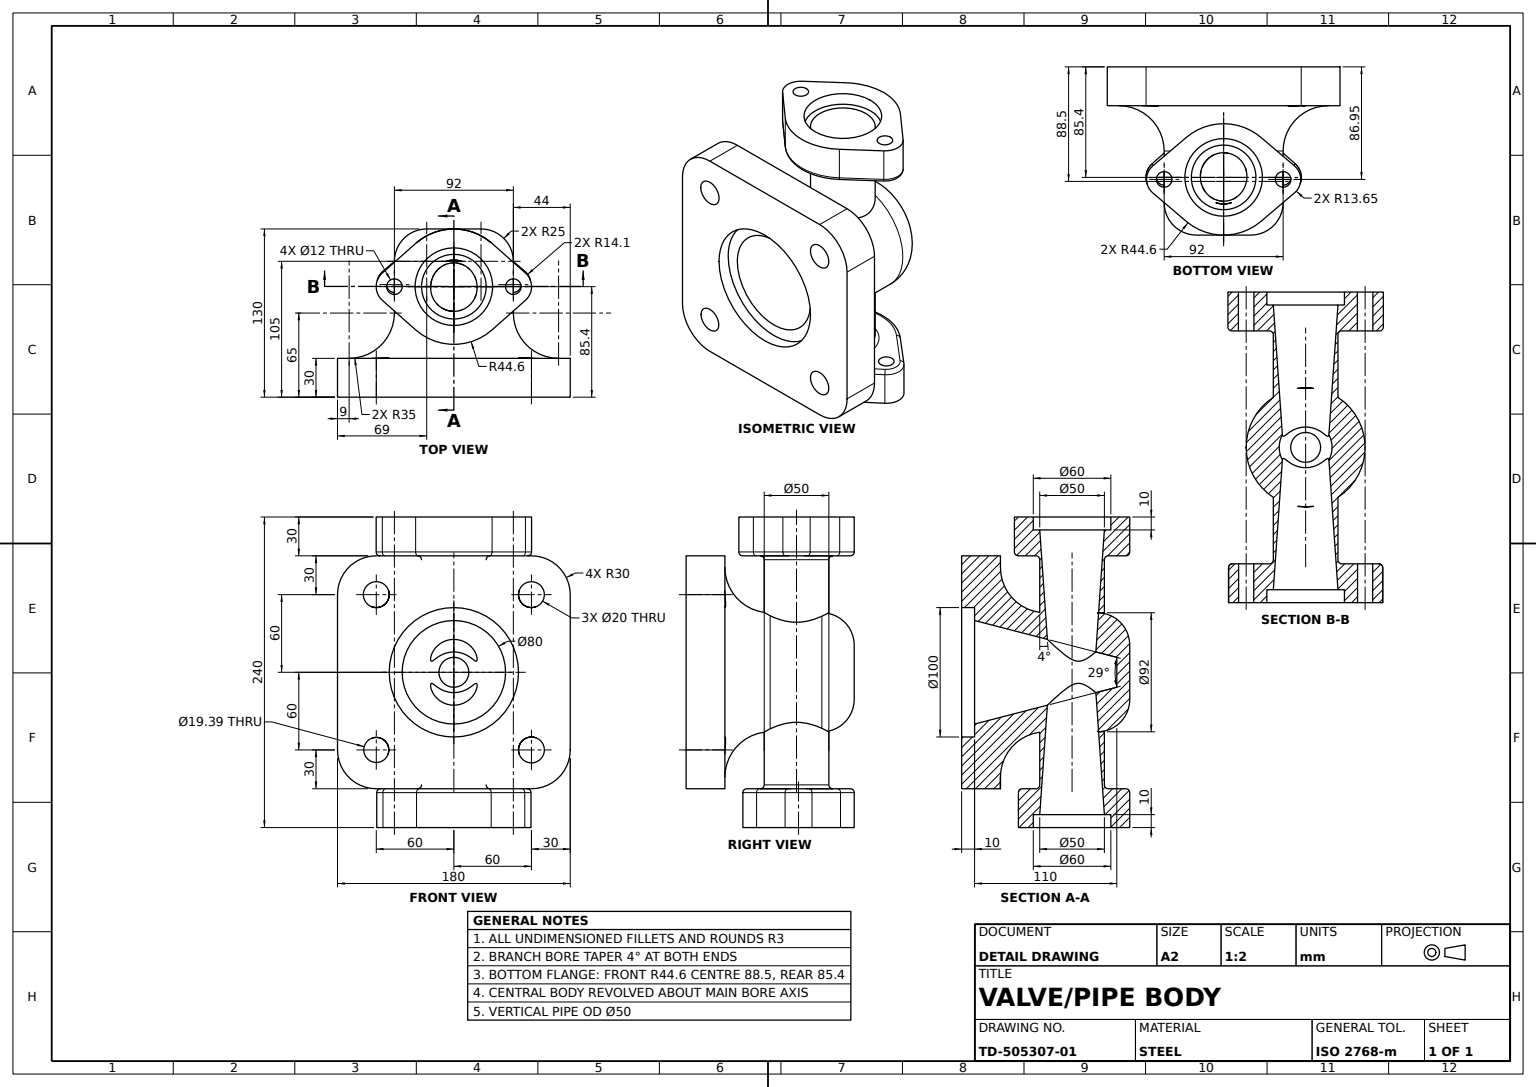
SolidWorks part; units mm, degrees
material "Plain Carbon Steel"
ref_plane "Front Plane" through (0, 0, 0) normal (0, 0, 1) x (1, 0, 0)
ref_plane "Top Plane" through (0, 0, 0) normal (0, 1, 0) x (1, 0, 0)
ref_plane "Right Plane" through (0, 0, 0) normal (1, 0, 0) x (0, 0, -1)
sketch "Square Flange Sketch" plane through (0, 0, 0) normal (0, 0, 1) x (1, 0, 0)
  line L1 (-90, 90) -> (90, 90)
  line L2 (-90, 90) -> (-90, -90)
  line L3 (-90, -90) -> (90, -90)
  line L4 (90, 90) -> (90, -90)
  line L5 (-90, 90) -> (90, -90) construction
  line L6 (-90, -90) -> (90, 90) construction
  point P0 (0, 0)
  dimension "D1" = 180
  dimension "D2" = 180
extrude "Square Flange 180x180" add sketch "Square Flange Sketch" along normal blind 30
fillet "Flange Corner Fillets R30" radius 30 4 edges at (-90, -90, 15) (90, -90, 15) (-90, 90, 15) (90, 90, 15)
sketch "Tee Body Profile Sketch" plane through (0, 0, 0) normal (0, 1, 0) x (1, 0, 0)
  line L0 (0, 100) -> (0, 0) construction
  line L1 (0, 100) -> (21, 100)
  line L2 (46, 75) -> (46, 35)
  line L3 (0, 0) -> (81, 0)
  line L4 (0, 100) -> (0, 0)
  arc A0 (46, 75) -> (21, 100) centre (21, 75) ccw
  arc A1 (46, 35) -> (81, 0) centre (81, 35) ccw
  dimension "D2" = 25
  dimension "D4" = 35
  dimension "D1" = 100
  dimension "D3" = 46
revolve "Tee Body Revolve" add sketch "Tee Body Profile Sketch" angle 360 about L0
sketch "Oval Flange A Sketch" plane through (0, -90, 0) normal (0, -1, 0) x (1, 0, 0)
  line L0 (0, -113.6555) -> (0, 0) construction
  line L1 (73.4602, -56.9504) -> (-69.6808, -56.9504) construction
  line L2 (-28.8618, -24.4984) -> (-54.8334, -46.5436)
  line L3 (-54.8334, -67.3571) -> (-28.8618, -89.4023)
  line L4 (28.8618, -89.4023) -> (54.8334, -67.3571)
  line L5 (54.8334, -46.5436) -> (28.8618, -24.4984)
  arc A0 (28.8618, -89.4023) -> (-28.8618, -89.4023) centre (0, -55.4) cw
  arc A1 (-28.8618, -24.4984) -> (28.8618, -24.4984) centre (0, -58.5007) cw
  arc A2 (54.8334, -67.3571) -> (54.8334, -46.5436) centre (46, -56.9504) ccw
  arc A3 (-54.8334, -67.3571) -> (-54.8334, -46.5436) centre (-46, -56.9504) cw
  circle A4 centre (-46, -56.9504) radius 6
  circle A5 centre (46, -56.9504) radius 6
  point P10 (0, -113.9007)
  point P16 (67.0937, -56.9504)
  point P19 (-67.0937, -56.9504)
  point P20 (0, -100)
  dimension "D1" = 44.6
  dimension "D2" = 13.6502
  dimension "D5" = 12
  dimension "D6" = 12
  dimension "D3" = 92
  dimension "D4" = 100
extrude "Oval Flange A" add sketch "Oval Flange A Sketch" along normal blind 30 separate body
sketch "Oval Flange B Sketch" plane through (0, 90, 0) normal (0, 1, 0) x (1, 0, 0)
  line L0 (0, 109.9701) -> (0, 0) construction
  line L1 (110.9056, 55.4) -> (-68.1303, 55.4) construction
  line L2 (29.5717, 88.7867) -> (55.3489, 65.955)
  line L3 (55.3489, 44.845) -> (29.5717, 22.0133)
  line L4 (-29.5717, 22.0133) -> (-55.3489, 44.845)
  line L5 (-55.3489, 65.955) -> (-29.5717, 88.7867)
  arc A0 (29.5717, 22.0133) -> (-29.5717, 22.0133) centre (0, 55.4) cw
  arc A1 (-29.5717, 88.7867) -> (29.5717, 88.7867) centre (0, 55.4) cw
  arc A2 (55.3489, 44.845) -> (55.3489, 65.955) centre (46, 55.4) ccw
  arc A3 (-55.3489, 65.955) -> (-55.3489, 44.845) centre (-46, 55.4) ccw
  circle A4 centre (-46, 55.4) radius 6
  circle A5 centre (46, 55.4) radius 6
  point P11 (0, -4.1794)
  point P14 (0, 114.9794)
  point P17 (67.2656, 55.4)
  point P20 (-67.2656, 55.4)
  point P25 (0, 100)
  dimension "D1" = 44.6
  dimension "D2" = 14.1
  dimension "D5" = 12
  dimension "D6" = 12
  dimension "D3" = 100
  dimension "D4" = 92
extrude "Oval Flange B" add sketch "Oval Flange B Sketch" along normal blind 30 separate body
sketch "Flange B Counterbore Sketch" plane through (0, 120, 0) normal (0, 1, 0) x (1, 0, 0)
  circle A0 centre (0, 55.4) radius 30
  dimension "D1" = 60
extrude "Flange B Counterbore Ø60" cut sketch "Flange B Counterbore Sketch" against normal blind 10
sketch "Flange A Counterbore Sketch" plane through (0, -120, 0) normal (0, -1, 0) x (1, 0, 0)
  circle A0 centre (0, -55.4) radius 30
  dimension "D1" = 60
extrude "Flange A Counterbore Ø60" cut sketch "Flange A Counterbore Sketch" against normal blind 10
sketch "Main Port Counterbore Sketch" plane through (0, 0, 30) normal (0, 0, 1) x (1, 0, 0)
  circle A0 centre (0, 0) radius 50
  dimension "D1" = 100
extrude "Main Port Counterbore Ø100" cut sketch "Main Port Counterbore Sketch" against normal blind 10
sketch "Main Bore Sketch" plane through (0, 0, 20) normal (0, 0, 1) x (1, 0, 0)
  circle A0 centre (0, 0) radius 40
  dimension "D1" = 80
extrude "Main Tapered Bore Ø80" cut sketch "Main Bore Sketch" against normal blind 110 draft 14.5
sketch "Branch Neck B Sketch" plane through (0, 90, 0) normal (0, -1, 0) x (1, 0, 0)
  circle A0 centre (0, -55.4) radius 25
  dimension "D1" = 50
extrude "Branch Neck B Ø50" add sketch "Branch Neck B Sketch" along normal up to surface (44 mm away)
sketch "Branch Neck A Sketch" plane through (0, -90, 0) normal (0, 1, 0) x (1, 0, 0)
  circle A0 centre (0, 55.4) radius 25
  dimension "D1" = 50
extrude "Branch Neck A Ø50" add sketch "Branch Neck A Sketch" along normal up to surface (44 mm away)
sketch "Branch Bore B Sketch" plane through (0, 110, 0) normal (0, 1, 0) x (1, 0, 0)
  circle A0 centre (0, 55.4) radius 25
  dimension "D1" = 50
extrude "Branch Tapered Bore B Ø50" cut sketch "Branch Bore B Sketch" against normal blind 110 draft 4
sketch "Branch Bore A Sketch" plane through (0, -110, 0) normal (0, -1, 0) x (1, 0, 0)
  circle A0 centre (0, -55.4) radius 25
  dimension "D1" = 50
extrude "Branch Tapered Bore A Ø50" cut sketch "Branch Bore A Sketch" against normal blind 110 draft 4
fillet "Oval Flange Fillets R3" radius 3 16 edges at (-41.8476, -90, -78.3797) (-59.6502, -90, -56.9504) (-41.8476, -90, -35.521) (0, -90, -13.9007) (41.8476, -90, -35.521) (59.6502, -90, -56.9504) (41.8476, -90, -78.3797) (42.4603, 90, -77.3708) (60.1, 90, -55.4) (42.4603, 90, -33.4292) (0, 90, -10.8) (-42.4603, 90, -33.4292) (-60.1, 90, -55.4) (-42.4603, 90, -77.3708) (0, -90, -100) (0, 90, -100)
fillet "Branch Neck Fillets R3" radius 3 2 edges at (0, -90, -30.4) (0, 90, -80.4)
sketch "Relief Cut 12x12 Sketch" plane through (0, 0, 30) normal (0, 0, 1) x (1, 0, 0)
  line L0 (0, 90) -> (0, -90) construction
  line L1 (-27.5826, 90) -> (27.5826, 90) construction
  line L2 (-60, -90) -> (60, -90) construction
  line L3 (90, 0) -> (-90, 0) construction
  line L4 (90, -60) -> (90, 60) construction
  line L5 (-90, 60) -> (-90, -60) construction
  circle A0 centre (-60, 60) radius 6
  circle A1 centre (60, 60) radius 6
  circle A2 centre (60, -60) radius 6
  circle A3 centre (-60, -60) radius 6
  dimension "D1" = 12
  dimension "D2" = 12
extrude "Relief Cut 12x12" cut sketch "Relief Cut 12x12 Sketch" against normal blind 15
sketch "Relief Cut 20x20 Sketch" plane through (0, 0, 30) normal (0, 0, 1) x (1, 0, 0)
  circle A0 centre (-60, 60) radius 10
  circle A1 centre (60, 60) radius 10
  circle A2 centre (-60, -60) radius 9.6926
  circle A3 centre (60, -60) radius 10
  dimension "D1" = 20
  dimension "D2" = 20
  dimension "D3" = 20
  dimension "D4" = 19.3852
extrude "Relief Cut 20x20" cut sketch "Relief Cut 20x20 Sketch" against normal blind 35
